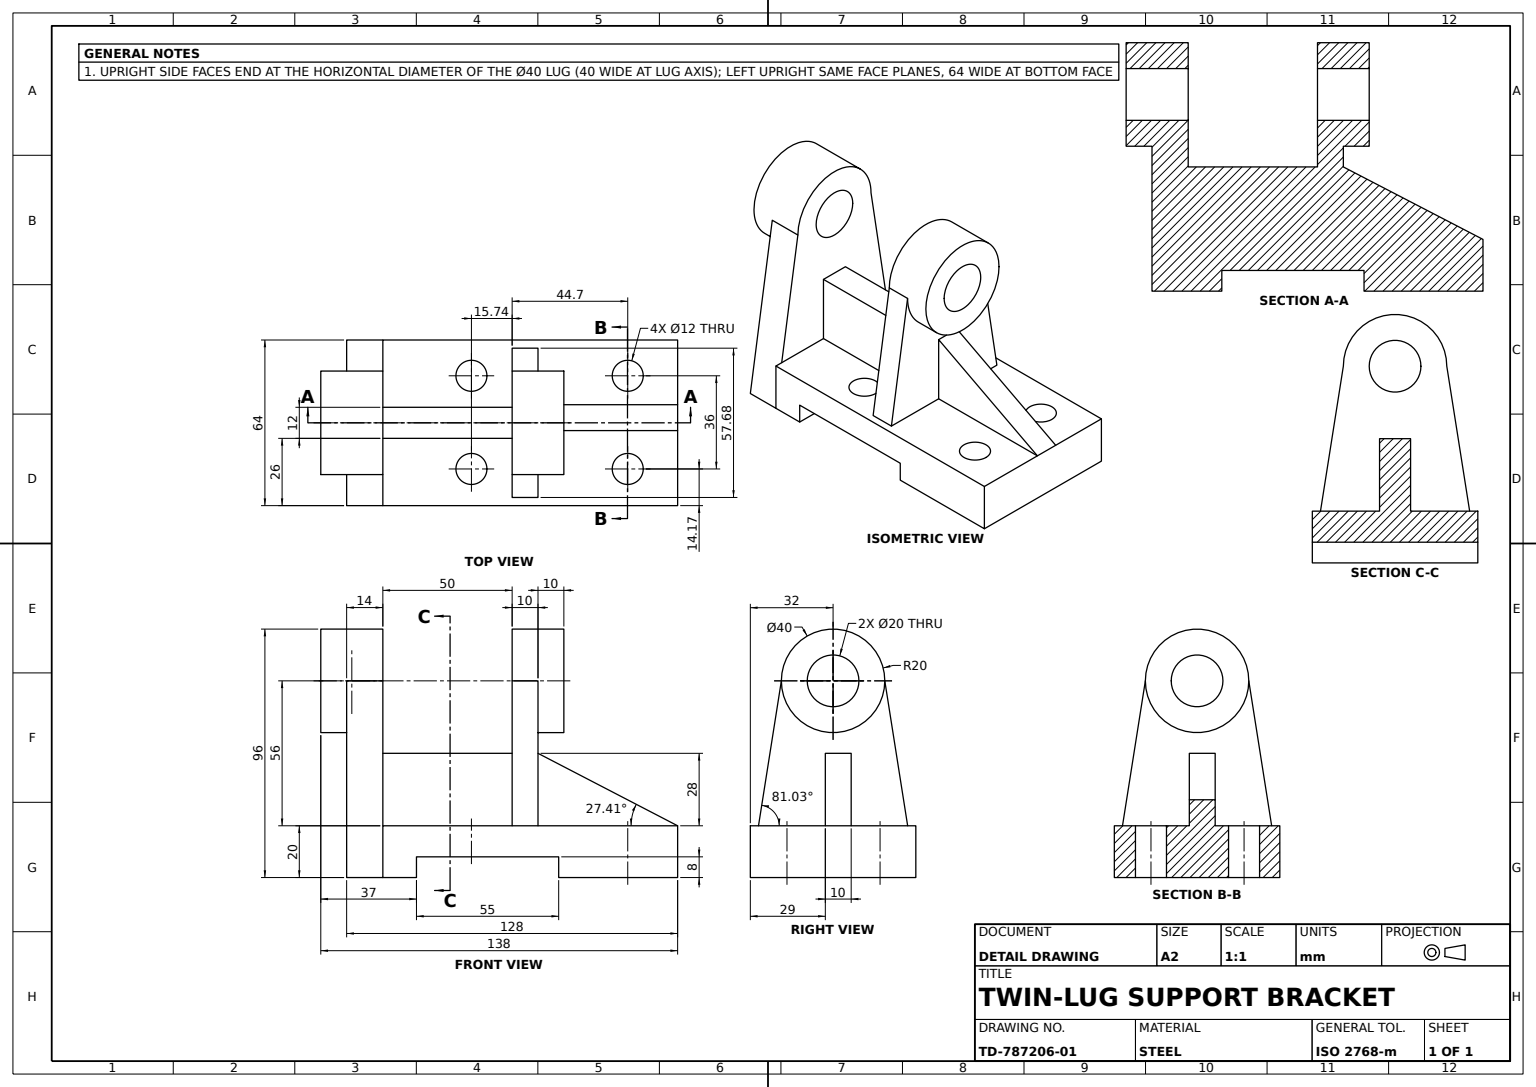
from build123d import *

# Parameters (mm, degrees)
BASE_PROFILE_SKETCH_W           = 128
BASE_PROFILE_SKETCH_H           = 20
BASE_PLATE_DEPTH                = 64
UNDERSIDE_RELIEF_CUT_DEPTH      = 92.060419503
UNDERSIDE_RELIEF_CUT_DEPTH_BACK = 64
UNDERSIDE_RELIEF_SKETCH_W       = 55
UNDERSIDE_RELIEF_SKETCH_H       = 8
FIRST_UPRIGHT_SKETCH_W          = 14
FIRST_UPRIGHT_SKETCH_H          = 64
FIRST_UPRIGHT_DEPTH             = 56
FIRST_TRUNNION_BOSS_DEPTH       = 10
FIRST_TRUNNION_BOSS_DEPTH_BACK  = 14
FIRST_TRUNNION_BOSS_SKETCH_R    = 20
FIRST_TRUNNION_BOSS_SKETCH_R_2  = 10
FIRST_TRUNNION_BORE_DEPTH       = 14
FIRST_UPRIGHT_TAPER_CUT_DEPTH   = 14
CENTER_BLOCK_DEPTH              = 28
SECOND_TRUNNION_BOSS_SKETCH_R   = 20
SECOND_TRUNNION_BOSS_SKETCH_R_2 = 10
SECOND_TRUNNION_BOSS_DEPTH      = 20
SECOND_UPRIGHT_DEPTH            = 10
SECOND_TRUNNION_BORE_DEPTH      = 10
GUSSET_RIB_REACH                = 120.44
GUSSET_RIB_SKETCH_WALL_W        = 299.707341614
GUSSET_RIB_SKETCH_WALL_H        = 10
BASE_MOUNTING_HOLES_SKETCH_R    = 6
BASE_MOUNTING_HOLES_DEPTH       = 124.887045328


with BuildPart() as part:
    # Base Profile Sketch → Base Plate (new body)
    with BuildSketch(Plane.XY):
        Rectangle(BASE_PROFILE_SKETCH_W, BASE_PROFILE_SKETCH_H)
    extrude(amount=BASE_PLATE_DEPTH)

    # Underside Relief Sketch → Underside Relief Cut (cut, two sides: drawn at the far end of the back side and taken through both)
    with BuildSketch(Plane.XY.offset(-UNDERSIDE_RELIEF_CUT_DEPTH_BACK)):
        with Locations((-9.5, -6)):
            Rectangle(UNDERSIDE_RELIEF_SKETCH_W, UNDERSIDE_RELIEF_SKETCH_H)
    extrude(amount=UNDERSIDE_RELIEF_CUT_DEPTH + UNDERSIDE_RELIEF_CUT_DEPTH_BACK, mode=Mode.SUBTRACT)

    # First Upright Sketch → First Upright (add)
    with BuildSketch(Plane(origin=(0, 10, 0), x_dir=(1, 0, 0), z_dir=(0, 1, 0))):
        with Locations((-57, -32)):
            Rectangle(FIRST_UPRIGHT_SKETCH_W, FIRST_UPRIGHT_SKETCH_H)
    extrude(amount=FIRST_UPRIGHT_DEPTH)

    # First Trunnion Boss Sketch → First Trunnion Boss (add, two sides: drawn at the far end of the back side and taken through both)
    with BuildSketch(Plane.ZY.offset(64).offset(-FIRST_TRUNNION_BOSS_DEPTH_BACK)):
        with Locations((32, 66)):
            Circle(FIRST_TRUNNION_BOSS_SKETCH_R)
        with Locations((32, 66)):
            Circle(FIRST_TRUNNION_BOSS_SKETCH_R_2, mode=Mode.SUBTRACT)
    extrude(amount=FIRST_TRUNNION_BOSS_DEPTH + FIRST_TRUNNION_BOSS_DEPTH_BACK)

    # First Trunnion Bore Sketch → First Trunnion Bore (cut)
    with BuildSketch(Plane.ZY.offset(64)):
        with BuildLine():
            Line((42, 66), (22, 66))
            ThreePointArc((22, 66), (32, 56), (42, 66))
        make_face()
    extrude(amount=-FIRST_TRUNNION_BORE_DEPTH, mode=Mode.SUBTRACT)

    # First Upright Taper Sketch → First Upright Taper Cut (cut)
    with BuildSketch(Plane.ZY.offset(64)):
        Polygon((12, 66), (0, -10), (0, 66), align=None)
        Polygon((64, -10), (52, 66), (64, 66), align=None)
    extrude(amount=-FIRST_UPRIGHT_TAPER_CUT_DEPTH, mode=Mode.SUBTRACT)

    # Center Block Sketch → Center Block (add)
    with BuildSketch(Plane(origin=(0, 10, 0), x_dir=(1, 0, 0), z_dir=(0, 1, 0))):
        Polygon((-50, -32), (-50, -26), (0, -26), (0, -38), (-50, -38), align=None)
    extrude(amount=CENTER_BLOCK_DEPTH)



with BuildPart() as body_2:
    # Second Trunnion Boss Sketch → Second Trunnion Boss (new body)
    with BuildSketch(Plane(origin=(0, 0, 0), x_dir=(0, 0, -1), z_dir=(1, 0, 0))):
        with Locations(Location((-32, 66, 0), (0, 0, 180))):
            Circle(SECOND_TRUNNION_BOSS_SKETCH_R)
        with Locations(Location((-32, 66, 0), (0, 0, 180))):
            Circle(SECOND_TRUNNION_BOSS_SKETCH_R_2, mode=Mode.SUBTRACT)
    extrude(amount=SECOND_TRUNNION_BOSS_DEPTH)


with BuildPart() as part_1:
    add(part.part)

    add(body_2.part)  # Second Upright merges body 2
    # Second Upright Sketch → Second Upright (add)
    with BuildSketch(Plane(origin=(0, 0, 0), x_dir=(0, 0, -1), z_dir=(1, 0, 0))):
        Polygon((-52, 66), (-60.842105263, 10), (-3.157894737, 10), (-12, 66), align=None)
    extrude(amount=SECOND_UPRIGHT_DEPTH)

    # Second Trunnion Bore Sketch → Second Trunnion Bore (cut)
    with BuildSketch(Plane(origin=(0, 0, 0), x_dir=(0, 0, -1), z_dir=(1, 0, 0))):
        with BuildLine():
            Line((-22, 66), (-42, 66))
            ThreePointArc((-42, 66), (-32, 56), (-22, 66))
        make_face()
    extrude(amount=SECOND_TRUNNION_BORE_DEPTH, mode=Mode.SUBTRACT)

    # Gusset Rib Sketch wall → Gusset Rib (add, up to next)
    with BuildSketch(Plane(origin=(37, 24, 30), x_dir=(0.887754531449, -0.460317164455, 0), z_dir=(0.460317164455, 0.887754531449, 0)), mode=Mode.PRIVATE) as gusset_rib_sk1:
        Rectangle(GUSSET_RIB_SKETCH_WALL_W, GUSSET_RIB_SKETCH_WALL_H)
    gusset_rib_tool1 = extrude(gusset_rib_sk1.sketch, amount=-GUSSET_RIB_REACH, mode=Mode.PRIVATE) - part_1.part
    add(gusset_rib_tool1.solids().sort_by_distance((37, 24, 30))[0])

    # Base Mounting Holes Sketch → Base Mounting Holes (cut, through all)
    with BuildSketch(Plane(origin=(0, 10, 0), x_dir=(1, 0, 0), z_dir=(0, 1, 0))):
        with Locations(Location((-15.743786959, -13.828319493, 0), (0, 0, 180))):
            Circle(BASE_MOUNTING_HOLES_SKETCH_R)
        with Locations(Location((-15.743786959, -49.828319493, 0), (0, 0, 180))):
            Circle(BASE_MOUNTING_HOLES_SKETCH_R)
        with Locations(Location((44.704140343, -13.828319493, 0), (0, 0, 180))):
            Circle(BASE_MOUNTING_HOLES_SKETCH_R)
        with Locations(Location((44.704140343, -49.828319493, 0), (0, 0, 180))):
            Circle(BASE_MOUNTING_HOLES_SKETCH_R)
    extrude(amount=-BASE_MOUNTING_HOLES_DEPTH, mode=Mode.SUBTRACT)


solid = part_1.part
